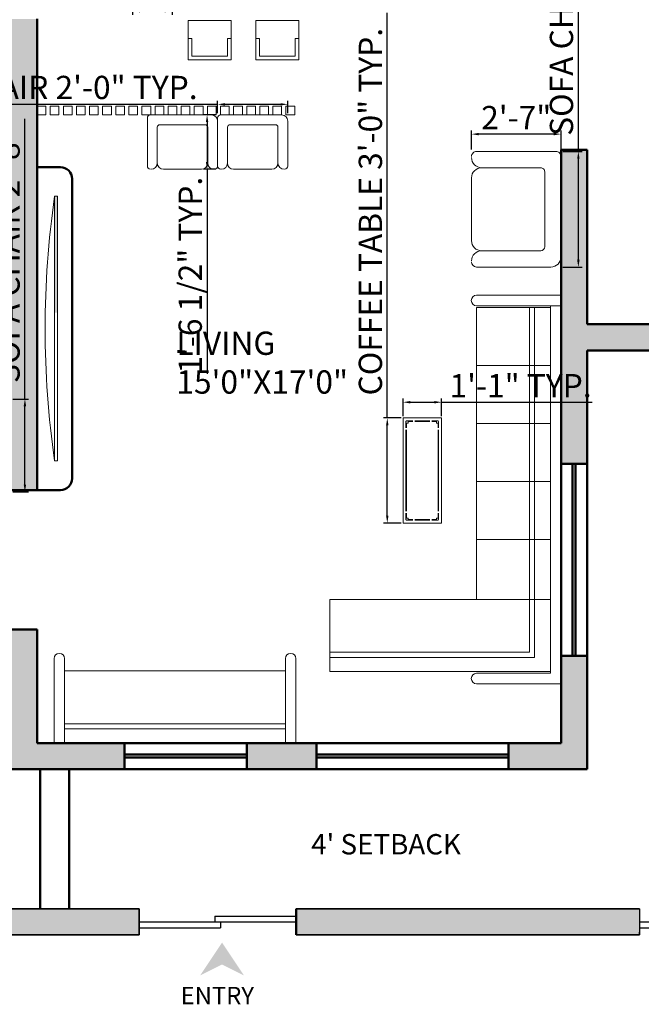
# Model space of a CAD drawing. Units: inches. Extents: x 2442 to 3851, y 589 to 2836.
# Tile 5 of 22: x 2698 to 2911, y 1378 to 1717. Entities that reach past the tile are written whole.
import ezdxf

# ---------------------------------------------------------------- set-up
doc = ezdxf.new("R2010")
doc.units = ezdxf.units.IN
for name, color, linetype, lineweight in [('A-ANNO-DIMS', 2, 'Continuous', 18), ('A-ANNO-SYMB', 1, 'Continuous', 18), ('A-ANNO-TEXT', 7, 'Continuous', 18), ('A-AREA-IDEN', 7, 'Continuous', 18), ('A-FURN', 8, 'Continuous', 18), ('A-GLAZ', 1, 'Continuous', 25), ('A-WALL', 7, 'Continuous', 50), ('A-WALL-PATT', 8, 'Continuous', 13), ('C-PROP', 7, 'Continuous', 35)]:
    doc.layers.add(name, color=color, linetype=linetype, lineweight=lineweight)
doc.styles.get("Standard").update_dxf_attribs({"font": 'arial.ttf'})
doc.dimstyles.new('ISO-25', dxfattribs={"dimtxt": 8, "dimasz": 2.5, "dimexe": 1.25, "dimexo": 0.625, "dimtad": 1, "dimlunit": 3, "dimtxsty": 'Standard', "dimcen": 2.5, "dimadec": 0, "dimazin": 0, "dimtfac": 1, "dimtmove": 0, "dimatfit": 3, "dimfxl": 1, "dimarcsym": 0})

# ---------------------------------------------------------------- blocks, each defined once
blk = doc.blocks.new('sofa-27')
at = {"color": 0, "linetype": 'ByBlock'}
for p, q in [((0.0945, 0.5198), (0.459, 0.5198)), ((-0.0591, 0.0591), (-0.0591, 0.4902)), ((0.0354, 0.1181), (0.0354, 0.4607)), ((0.518, 0.1181), (0.518, 0.4607)), ((0.6125, 0.0295), (0.6125, 0.4902)), ((0.4944, 0.0945), (0.0591, 0.0945)), ((0.583, 0), (0, 0))]:
    blk.add_line(p, q, dxfattribs=at)
for centre, radius, start, end in [((-0.0295, 0.4902), 0.0295, 90, 180), ((-0.0236, 0.4607), 0.0591, 360, 90), ((0.0945, 0.4607), 0.0591, 90, 180), ((0.459, 0.4607), 0.0591, 0, 90), ((0.5771, 0.4607), 0.0591, 90, 180), ((0.583, 0.4902), 0.0295, 0, 90), ((0.0591, 0.1181), 0.0236, 180, 270), ((0.4944, 0.1181), 0.0236, 270, 0), ((0, 0.0591), 0.0591, 180, 270), ((0.583, 0.0295), 0.0295, 270, 0)]:
    blk.add_arc(centre, radius, start, end, dxfattribs=at)
blk = doc.blocks.new('TABLE-30A')
at = {"color": 0, "linetype": 'ByBlock'}
for p, q in [((0, 0), (0, 0.55)), ((0, 0.55), (1.5, 0.55)), ((0.051, 0.508), (0.042, 0.499)), ((0.042, 0.499), (0.042, 0.478)), ((0.042, 0.478), (0.072, 0.478)), ((0.042, 0.478), (0.042, 0.41)), ((0.072, 0.508), (0.051, 0.508)), ((0.051, 0.478), (0.051, 0.41)), ((0.072, 0.478), (0.072, 0.508)), ((0.072, 0.508), (0.14, 0.508)), ((0.072, 0.499), (0.14, 0.499)), ((1.331, 0.508), (0.169, 0.508)), ((1.331, 0.499), (0.169, 0.499)), ((1.428, 0.508), (1.36, 0.508)), ((1.428, 0.499), (1.36, 0.499)), ((1.428, 0.508), (1.428, 0.478)), ((1.449, 0.508), (1.428, 0.508)), ((1.428, 0.478), (1.458, 0.478)), ((1.458, 0.499), (1.449, 0.508)), ((1.449, 0.478), (1.449, 0.41)), ((1.458, 0.478), (1.458, 0.499)), ((1.458, 0.478), (1.458, 0.41)), ((1.5, 0.55), (1.5, 0)), ((0.042, 0.169), (0.042, 0.381)), ((0.051, 0.169), (0.051, 0.381)), ((1.449, 0.381), (1.449, 0.169)), ((1.458, 0.381), (1.458, 0.169)), ((1.5, 0), (0, 0)), ((0.042, 0.072), (0.042, 0.14)), ((0.042, 0.072), (0.042, 0.051)), ((0.072, 0.072), (0.042, 0.072)), ((0.042, 0.051), (0.051, 0.042)), ((0.051, 0.072), (0.051, 0.14)), ((0.051, 0.042), (0.072, 0.042)), ((0.072, 0.042), (0.072, 0.072)), ((0.072, 0.051), (0.14, 0.051)), ((0.072, 0.042), (0.14, 0.042)), ((0.169, 0.051), (1.331, 0.051)), ((0.169, 0.042), (1.331, 0.042)), ((1.428, 0.051), (1.36, 0.051)), ((1.428, 0.042), (1.36, 0.042)), ((1.428, 0.072), (1.428, 0.042)), ((1.458, 0.072), (1.428, 0.072)), ((1.428, 0.042), (1.449, 0.042)), ((1.449, 0.072), (1.449, 0.14)), ((1.449, 0.042), (1.458, 0.051)), ((1.458, 0.072), (1.458, 0.14)), ((1.458, 0.051), (1.458, 0.072))]:
    blk.add_line(p, q, dxfattribs=at)
blk = doc.blocks.new('*U26')
at = {"linetype": 'ByBlock'}
blk.add_lwpolyline([(-1.5, -1.5), (1.5, -1.5), (1.5, 1.5), (-1.5, 1.5)], close=True, dxfattribs=at)
blk = doc.blocks.new('*U27')
at = {"layer": 'A-FURN', "color": 0, "linetype": 'ByBlock', "lineweight": -2, "transparency": 16777216}
for p in [(0, 0), (4.5, 0), (9, 0), (13.5, 0), (18, 0), (22.5, 0), (27, 0), (31.5, 0), (36, 0), (40.5, 0), (45, 0), (49.5, 0), (54, 0), (58.5, 0), (63, 0), (67.5, 0), (72, 0), (76.5, 0), (81, 0), (85.5, 0)]:
    blk.add_blockref('*U26', p, dxfattribs=at)
blk = doc.blocks.new('CHAIR-DINING')
for p, q in [((0, 14.84), (13.57, 14.84)), ((0, 0), (0, 14.84)), ((1.28, 13.56), (7.42, 13.56)), ((1.28, 1.32), (1.28, 13.56)), ((7.42, 13.56), (7.42, 14.84)), ((13.57, 0), (13.57, 14.84)), ((0, 0), (13.57, 0)), ((7.42, 1.32), (1.28, 1.32)), ((7.42, 0), (7.42, 1.32))]:
    blk.add_line(p, q)
blk = doc.blocks.new('SOFA-L')
for p, q in [((79.48, 133.62), (50.46, 133.62)), ((79.48, 0), (79.48, 133.62)), ((79.48, 129.99), (50.46, 129.99)), ((50.46, 129.38), (50.46, 29.02)), ((75.86, 129.38), (50.46, 129.38)), ((75.86, 129.38), (50.46, 129.38)), ((75.86, 3.63), (75.86, 129.99)), ((75.86, 29.02), (0, 29.02)), ((0, 4.23), (0, 29.02)), ((75.86, 4.23), (0, 4.23)), ((50.46, 3.63), (75.86, 3.63)), ((50.46, 0), (79.48, 0))]:
    blk.add_line(p, q)
for centre in [(50.46, 131.8), (50.46, 1.81)]:
    blk.add_arc(centre, 1.81, 90, 270)
blk = doc.blocks.new('SOFA-3SEAT')
for p, q in [((0, 29.02), (0, 0)), ((3.63, 0), (3.63, 29.02)), ((79.48, 29.02), (79.48, 0)), ((83.11, 29.02), (83.11, 0)), ((83.11, 0), (0, 0))]:
    blk.add_line(p, q)
for centre in [(1.81, 29.02), (81.3, 29.02)]:
    blk.add_arc(centre, 1.81, 0, 180)
blk = doc.blocks.new('*D149')
at = {"layer": 'A-ANNO-DIMS', "color": 0, "lineweight": -2, "transparency": 16777216}
for p, q in [((2736.38, 1721.15), (2736.38, 1718.3)), ((2749.95, 1721.15), (2749.95, 1718.3)), ((2738.88, 1719.55), (2747.45, 1719.55)), ((2749.95, 1719.55), (2820.35, 1719.55))]:
    blk.add_line(p, q, dxfattribs=at)
at = {"layer": 'A-ANNO-DIMS', "color": 0, "transparency": 16777216}
for points in [[(2738.88, 1719.96), (2738.88, 1719.13), (2736.38, 1719.55)], [(2747.45, 1719.96), (2747.45, 1719.13), (2749.95, 1719.55)]]:
    blk.add_solid(points, dxfattribs=at)
at = {"layer": 'Defpoints', "color": 0, "transparency": 16777216}
for p in [(2736.38, 1721.77), (2749.95, 1721.77), (2749.95, 1719.55)]:
    blk.add_point(p, dxfattribs=at)
at = {"layer": 'A-ANNO-DIMS', "color": 0, "transparency": 16777216, "insert": (2786.4, 1724.31), "char_height": 8, "attachment_point": 5}
blk.add_mtext('1\'-1 1/2" TYP.', dxfattribs=at)
blk = doc.blocks.new('*D150')
at = {"layer": 'A-ANNO-DIMS', "color": 0, "lineweight": -2, "transparency": 16777216}
for p, q in [((2699.39, 1586.16), (2699.39, 1682.55)), ((2695.22, 1586.16), (2700.64, 1586.16)), ((2699.39, 1556.72), (2699.39, 1583.66)), ((2695.22, 1554.22), (2700.64, 1554.22))]:
    blk.add_line(p, q, dxfattribs=at)
at = {"layer": 'A-ANNO-DIMS', "color": 0, "transparency": 16777216}
for points in [[(2698.97, 1583.66), (2699.81, 1583.66), (2699.39, 1586.16)], [(2698.97, 1556.72), (2699.81, 1556.72), (2699.39, 1554.22)]]:
    blk.add_solid(points, dxfattribs=at)
at = {"layer": 'Defpoints', "color": 0, "transparency": 16777216}
for p in [(2694.6, 1586.16), (2699.39, 1586.16), (2694.6, 1554.22)]:
    blk.add_point(p, dxfattribs=at)
at = {"layer": 'A-ANNO-DIMS', "color": 0, "transparency": 16777216, "insert": (2694.63, 1635.61), "char_height": 8, "attachment_point": 5, "rotation": 90}
blk.add_mtext('SOFA CHAIR 2\'-8"', dxfattribs=at)
blk = doc.blocks.new('*D152')
at = {"layer": 'A-ANNO-DIMS', "color": 0, "lineweight": -2, "transparency": 16777216}
for p, q in [((2889.56, 1671.28), (2889.56, 1786.31)), ((2884.22, 1671.28), (2890.81, 1671.28)), ((2889.56, 1634.03), (2889.56, 1668.78)), ((2884.22, 1631.53), (2890.81, 1631.53))]:
    blk.add_line(p, q, dxfattribs=at)
at = {"layer": 'A-ANNO-DIMS', "color": 0, "transparency": 16777216}
for points in [[(2889.14, 1668.78), (2889.98, 1668.78), (2889.56, 1671.28)], [(2889.14, 1634.03), (2889.98, 1634.03), (2889.56, 1631.53)]]:
    blk.add_solid(points, dxfattribs=at)
at = {"layer": 'Defpoints', "color": 0, "transparency": 16777216}
for p in [(2883.6, 1671.28), (2889.56, 1671.28), (2883.6, 1631.53)]:
    blk.add_point(p, dxfattribs=at)
at = {"layer": 'A-ANNO-DIMS', "color": 0, "transparency": 16777216, "insert": (2884.79, 1730.04), "char_height": 8, "attachment_point": 5, "rotation": 90}
blk.add_mtext('SOFA CHAIR 3\'-3 1/2"', dxfattribs=at)
blk = doc.blocks.new('*D153')
at = {"layer": 'A-ANNO-DIMS', "color": 0, "lineweight": -2, "transparency": 16777216}
for p, q in [((2852.84, 1671.9), (2852.84, 1678.49)), ((2881.1, 1677.24), (2855.34, 1677.24)), ((2883.6, 1671.9), (2883.6, 1678.49))]:
    blk.add_line(p, q, dxfattribs=at)
at = {"layer": 'A-ANNO-DIMS', "color": 0, "transparency": 16777216}
for points in [[(2855.34, 1677.66), (2855.34, 1676.82), (2852.84, 1677.24)], [(2881.1, 1677.66), (2881.1, 1676.82), (2883.6, 1677.24)]]:
    blk.add_solid(points, dxfattribs=at)
at = {"layer": 'Defpoints', "color": 0, "transparency": 16777216}
for p in [(2852.84, 1677.24), (2852.84, 1671.28), (2883.6, 1671.28)]:
    blk.add_point(p, dxfattribs=at)
at = {"layer": 'A-ANNO-DIMS', "color": 0, "transparency": 16777216, "insert": (2868.22, 1681.88), "char_height": 8, "attachment_point": 5}
blk.add_mtext('2\'-7"', dxfattribs=at)
blk = doc.blocks.new('*D154')
at = {"layer": 'A-ANNO-DIMS', "color": 0, "lineweight": -2, "transparency": 16777216}
for p, q in [((2765.6, 1687.48), (2641.71, 1687.48)), ((2765.6, 1684.49), (2765.6, 1688.73)), ((2787.22, 1687.48), (2768.1, 1687.48)), ((2789.72, 1684.49), (2789.72, 1688.73))]:
    blk.add_line(p, q, dxfattribs=at)
at = {"layer": 'A-ANNO-DIMS', "color": 0, "transparency": 16777216}
for points in [[(2768.1, 1687.9), (2768.1, 1687.07), (2765.6, 1687.48)], [(2787.22, 1687.9), (2787.22, 1687.07), (2789.72, 1687.48)]]:
    blk.add_solid(points, dxfattribs=at)
at = {"layer": 'Defpoints', "color": 0, "transparency": 16777216}
for p in [(2765.6, 1687.48), (2765.6, 1683.86), (2789.72, 1683.86)]:
    blk.add_point(p, dxfattribs=at)
at = {"layer": 'A-ANNO-DIMS', "color": 0, "transparency": 16777216, "insert": (2702.4, 1692.25), "char_height": 8, "attachment_point": 5}
blk.add_mtext('SOFA CHAIR 2\'-0" TYP.', dxfattribs=at)
blk = doc.blocks.new('*D155')
at = {"layer": 'A-ANNO-DIMS', "color": 0, "lineweight": -2, "transparency": 16777216}
for p, q in [((2764.97, 1683.86), (2760.73, 1683.86)), ((2761.98, 1681.36), (2761.98, 1667.69)), ((2764.97, 1665.19), (2760.73, 1665.19)), ((2761.98, 1665.19), (2761.98, 1594.79))]:
    blk.add_line(p, q, dxfattribs=at)
at = {"layer": 'A-ANNO-DIMS', "color": 0, "transparency": 16777216}
for points in [[(2761.56, 1681.36), (2762.4, 1681.36), (2761.98, 1683.86)], [(2761.56, 1667.69), (2762.4, 1667.69), (2761.98, 1665.19)]]:
    blk.add_solid(points, dxfattribs=at)
at = {"layer": 'Defpoints', "color": 0, "transparency": 16777216}
for p in [(2765.6, 1683.86), (2761.98, 1665.19), (2765.6, 1665.19)]:
    blk.add_point(p, dxfattribs=at)
at = {"layer": 'A-ANNO-DIMS', "color": 0, "transparency": 16777216, "insert": (2757.22, 1628.74), "char_height": 8, "attachment_point": 5, "rotation": 90}
blk.add_mtext('1\'-6 1/2" TYP.', dxfattribs=at)
blk = doc.blocks.new('*D166')
at = {"layer": 'A-ANNO-DIMS', "color": 0, "lineweight": -2, "transparency": 16777216}
for p, q in [((2823.9, 1579.64), (2823.9, 1719)), ((2828.69, 1579.64), (2822.65, 1579.64)), ((2823.9, 1546), (2823.9, 1577.14)), ((2828.69, 1543.5), (2822.65, 1543.5))]:
    blk.add_line(p, q, dxfattribs=at)
at = {"layer": 'A-ANNO-DIMS', "color": 0, "transparency": 16777216}
for points in [[(2823.48, 1577.14), (2824.31, 1577.14), (2823.9, 1579.64)], [(2823.48, 1546), (2824.31, 1546), (2823.9, 1543.5)]]:
    blk.add_solid(points, dxfattribs=at)
at = {"layer": 'Defpoints', "color": 0, "transparency": 16777216}
for p in [(2823.9, 1579.64), (2829.32, 1579.64), (2829.32, 1543.5)]:
    blk.add_point(p, dxfattribs=at)
at = {"layer": 'A-ANNO-DIMS', "color": 0, "transparency": 16777216, "insert": (2819.13, 1650.57), "char_height": 8, "attachment_point": 5, "rotation": 90}
blk.add_mtext('COFFEE TABLE 3\'-0" TYP.', dxfattribs=at)
blk = doc.blocks.new('*D167')
at = {"layer": 'A-ANNO-DIMS', "color": 0, "lineweight": -2, "transparency": 16777216}
for p, q in [((2829.32, 1580.26), (2829.32, 1586.31)), ((2831.82, 1585.06), (2840.07, 1585.06)), ((2842.57, 1580.26), (2842.57, 1586.31)), ((2842.57, 1585.06), (2894.33, 1585.06))]:
    blk.add_line(p, q, dxfattribs=at)
at = {"layer": 'A-ANNO-DIMS', "color": 0, "transparency": 16777216}
for points in [[(2831.82, 1585.47), (2831.82, 1584.64), (2829.32, 1585.06)], [(2840.07, 1585.47), (2840.07, 1584.64), (2842.57, 1585.06)]]:
    blk.add_solid(points, dxfattribs=at)
at = {"layer": 'Defpoints', "color": 0, "transparency": 16777216}
for p in [(2842.57, 1585.06), (2829.32, 1579.64), (2842.57, 1579.64)]:
    blk.add_point(p, dxfattribs=at)
at = {"layer": 'A-ANNO-DIMS', "color": 0, "transparency": 16777216, "insert": (2869.7, 1589.7), "char_height": 8, "attachment_point": 5}
blk.add_mtext('1\'-1" TYP.', dxfattribs=at)

msp = doc.modelspace()

# ---------------------------------------------------------------- hatches: boundary and pattern name
at = {"layer": 'A-ANNO-SYMB'}
h = msp.add_hatch(color=256, dxfattribs=at)
h.dxf.hatch_style = 1
h.paths.add_polyline_path([(2767.136, 1391.705), (2774.686, 1387.93), (2767.136, 1399.256), (2759.585, 1387.93)])
at = {"layer": 'A-FURN'}
h = msp.add_hatch(color=256, dxfattribs=at)
h.dxf.hatch_style = 1
h.paths.add_polyline_path([(2710.599, 1655.864), (2709.599, 1655.864), (2709.599, 1615.864), (2710.599, 1615.864)])
at = {"layer": 'A-WALL-PATT'}
h = msp.add_hatch(color=256, dxfattribs=at)
h.dxf.hatch_style = 1
h.paths.add_polyline_path([(2502.599, 1992.864), (2719.571, 1992.864), (2719.687, 1994.649), (2720.167, 1997.319), (2721.479, 1992.864), (2726.325, 1992.864), (2727.448, 1994.93), (2729.005, 1997.153), (2728.372, 1992.864), (2728.871, 1992.864), (2730.114, 1994.505), (2731.833, 1996.09), (2730.966, 1993.206), (2730.864, 1992.864), (2771.772, 1992.864), (2771.887, 1994.649), (2772.368, 1997.319), (2773.68, 1992.864), (2778.526, 1992.864), (2779.649, 1994.93), (2781.206, 1997.153), (2780.572, 1992.864), (2781.072, 1992.864), (2782.315, 1994.505), (2784.034, 1996.09), (2783.167, 1993.206), (2783.065, 1992.864), (2821.282, 1992.864), (2821.398, 1994.649), (2821.878, 1997.319), (2823.19, 1992.864), (2828.036, 1992.864), (2829.159, 1994.93), (2830.716, 1997.153), (2830.083, 1992.864), (2830.582, 1992.864), (2831.825, 1994.505), (2833.544, 1996.09), (2832.677, 1993.206), (2832.575, 1992.864), (2869.287, 1992.864), (2869.403, 1994.649), (2869.884, 1997.319), (2871.195, 1992.864), (2876.042, 1992.864), (2877.165, 1994.93), (2878.721, 1997.153), (2878.088, 1992.864), (2878.587, 1992.864), (2879.83, 1994.505), (2881.55, 1996.09), (2880.682, 1993.206), (2880.58, 1992.864), (2919.335, 1992.864), (2919.451, 1994.649), (2919.932, 1997.319), (2921.243, 1992.864), (2926.09, 1992.864), (2927.213, 1994.93), (2928.77, 1997.153), (2928.136, 1992.864), (2928.635, 1992.864), (2929.878, 1994.505), (2931.598, 1996.09), (2930.73, 1993.206), (2930.628, 1992.864), (2966.155, 1992.864), (2966.27, 1994.649), (2966.751, 1997.319), (2968.063, 1992.864), (2972.909, 1992.864), (2974.032, 1994.93), (2975.589, 1997.153), (2974.955, 1992.864), (2975.455, 1992.864), (2976.698, 1994.505), (2978.417, 1996.09), (2977.55, 1993.206), (2977.448, 1992.864), (3010.53, 1992.864), (3010.646, 1994.649), (3011.127, 1997.319), (3012.438, 1992.864), (3017.285, 1992.864), (3018.408, 1994.93), (3019.964, 1997.153), (3019.331, 1992.864), (3019.83, 1992.864), (3021.073, 1994.505), (3022.793, 1996.09), (3021.925, 1993.206), (3021.823, 1992.864), (3057.996, 1992.864), (3058.45, 1995.382), (3059.191, 1992.864), (3065.64, 1992.864), (3067.287, 1995.216), (3066.94, 1992.864), (3068.717, 1992.864), (3070.116, 1994.153), (3069.728, 1992.864), (3084.599, 1992.864), (3084.599, 1983.791), (3085.291, 1983.828), (3084.599, 1983.434), (3084.599, 1932.114), (3085.291, 1932.151), (3084.599, 1931.757), (3084.599, 1886.278), (3085.291, 1886.315), (3084.599, 1885.921), (3084.599, 1410.864), (3066.599, 1410.864), (3066.599, 1401.864), (3093.599, 1401.864), (3093.599, 2001.864), (2493.599, 2001.864), (2493.599, 1401.864), (2538.599, 1401.864), (2538.599, 1410.864), (2502.599, 1410.864)])
h.paths.add_polyline_path([(2738.599, 1410.864), (2547.599, 1410.864), (2547.599, 1401.864), (2738.599, 1401.864)], flags=17)
h.paths.add_polyline_path([(2910.599, 1410.864), (2792.599, 1410.864), (2792.599, 1401.864), (2910.599, 1401.864), (2910.599, 1402.864)], flags=17)
h = msp.add_hatch(color=256, dxfattribs=at)
h.dxf.hatch_style = 1
h.paths.add_polyline_path([(2799.599, 1467.864), (2775.599, 1467.864), (2775.599, 1458.864), (2799.599, 1458.864)])
h.paths.add_polyline_path([(2703.599, 1506.864), (2670.599, 1506.864), (2670.599, 1497.864), (2694.599, 1497.864), (2694.599, 1458.864), (2733.599, 1458.864), (2733.599, 1467.864), (2709.417, 1467.864), (2703.599, 1467.864)])
h.paths.add_polyline_path([(2604.599, 1506.864), (2593.599, 1506.864), (2593.599, 1497.864), (2604.599, 1497.864)])
h.paths.add_polyline_path([(2547.599, 1497.864), (2553.599, 1497.864), (2553.599, 1506.864), (2547.599, 1506.864), (2547.599, 1530.864), (2538.599, 1530.864), (2538.599, 1401.864), (2547.599, 1401.864)])
h.paths.add_polyline_path([(2547.599, 1683.864), (2538.599, 1683.864), (2538.599, 1578.864), (2547.599, 1578.864), (2547.599, 1602.864), (2694.599, 1602.864), (2694.599, 1554.864), (2703.599, 1554.864), (2703.599, 1716.864), (2694.599, 1716.864), (2694.599, 1611.864), (2547.599, 1611.864)])
h.paths.add_polyline_path([(2892.599, 1497.864), (2883.599, 1497.864), (2883.599, 1488.228), (2883.599, 1467.864), (2865.599, 1467.864), (2865.599, 1458.864), (2892.599, 1458.864)])
h.paths.add_polyline_path([(3048.599, 1722.864), (3039.599, 1722.864), (3039.599, 1716.864), (2937.599, 1716.864), (2937.599, 1710.864), (3039.599, 1710.864), (3039.599, 1685.364), (3048.599, 1685.364)])
h.paths.add_polyline_path([(3048.599, 1779.864), (3039.599, 1779.864), (3039.599, 1773.864), (2961.599, 1773.864), (2961.599, 1791.864), (2955.599, 1791.864), (2955.599, 1773.864), (2895.599, 1773.864), (2895.599, 1821.864), (2916.599, 1821.864), (2916.599, 1827.864), (2889.599, 1827.864), (2889.599, 1773.864), (2886.599, 1773.864), (2886.599, 1764.864), (2937.599, 1764.864), (2937.599, 1746.864), (2943.599, 1746.864), (2943.599, 1764.864), (2956.06, 1764.864), (3039.599, 1764.864), (3039.599, 1758.864), (3048.599, 1758.864)])
h.paths.add_polyline_path([(3048.599, 1827.864), (2976.475, 1827.864, -0.1284593), (2975.705, 1827.665), (2964.694, 1827.687, -0.1198794), (2963.972, 1827.864), (2946.599, 1827.864), (2946.599, 1821.864), (3039.599, 1821.864), (3039.599, 1815.864), (3048.599, 1815.864)])
h.paths.add_polyline_path([(3048.599, 1956.864), (3023.366, 1956.864), (3023.277, 1956.402), (3023.088, 1956.864), (3019.494, 1956.864), (3019.543, 1955.479), (3019.146, 1956.864), (3015.599, 1956.864), (3015.599, 1947.864), (3039.599, 1947.864), (3039.599, 1875.864), (3048.599, 1875.864), (3048.599, 1880.743), (3047.576, 1881.614), (3046.081, 1883.417), (3044.931, 1885.453), (3047.541, 1883.949), (3048.599, 1883.343), (3048.599, 1910.588), (3047.049, 1909.235), (3047.896, 1910.862), (3048.599, 1911.909), (3048.599, 1918.826), (3042.477, 1917.032), (3043.928, 1918.154), (3045.59, 1919.165), (3047.525, 1920.009), (3048.599, 1920.305), (3048.599, 1926.579), (3047.576, 1927.45), (3046.081, 1929.252), (3044.931, 1931.289), (3047.541, 1929.785), (3048.599, 1929.179)])
h.paths.add_polyline_path([(2967.599, 1956.864), (2932.171, 1956.864), (2932.082, 1956.402), (2931.893, 1956.864), (2928.299, 1956.864), (2928.348, 1955.479), (2927.951, 1956.864), (2898.599, 1956.864), (2898.599, 1947.864), (2967.599, 1947.864)])
h.paths.add_polyline_path([(2850.599, 1956.864), (2834.118, 1956.864), (2834.029, 1956.402), (2833.84, 1956.864), (2830.245, 1956.864), (2830.294, 1955.479), (2829.897, 1956.864), (2796.599, 1956.864), (2796.599, 1947.864), (2799.599, 1947.864), (2838.599, 1947.864), (2838.599, 1827.864), (2835.599, 1827.864), (2835.599, 1824.864), (2835.599, 1818.864), (2838.599, 1818.864), (2838.599, 1764.864), (2850.599, 1764.864), (2850.599, 1770.864), (2850.599, 1773.864), (2847.599, 1773.864), (2847.599, 1947.864), (2850.599, 1947.864)])
h.paths.add_polyline_path([(2700.599, 1947.864), (2730.599, 1947.864), (2730.599, 1956.864), (2700.599, 1956.864), (2700.599, 1992.864), (2691.599, 1992.864), (2691.599, 1932.864), (2670.599, 1932.864), (2670.599, 1923.864), (2691.599, 1923.864), (2691.599, 1818.864), (2799.599, 1818.864), (2799.599, 1827.864), (2700.599, 1827.864)])
h.paths.add_polyline_path([(2640.599, 1932.864), (2538.599, 1932.864), (2538.599, 1868.364), (2547.599, 1868.364), (2547.599, 1923.864), (2640.599, 1923.864), (2640.599, 1929.864)])
h.paths.add_polyline_path([(2547.599, 1820.364), (2538.599, 1820.364), (2538.599, 1731.864), (2547.599, 1731.864), (2547.599, 1755.864), (2694.599, 1755.864), (2694.599, 1752.864), (2697.599, 1752.864), (2703.599, 1752.864), (2703.599, 1764.864), (2547.599, 1764.864)])
h.paths.add_polyline_path([(2725.858, 1838.187), (2790.115, 1838.187), (2790.115, 1868.602), (2725.858, 1868.602)], flags=25)
h.paths.add_polyline_path([(2892.599, 1671.864), (2883.599, 1671.864), (2883.599, 1563.864), (2892.599, 1563.864), (2892.599, 1602.864), (3048.599, 1602.864), (3048.599, 1637.364), (3039.599, 1637.364), (3039.599, 1611.864), (2892.599, 1611.864)])

# ---------------------------------------------------------------- linework, layer by layer
at = {"layer": 'A-FURN'}
for p, q in [((2709.599, 1655.864), (2710.599, 1655.864)), ((2709.599, 1564.864), (2709.599, 1655.864)), ((2710.599, 1564.864), (2710.599, 1655.864)), ((2872.716, 1499.111), (2872.716, 1617.612)), ((2874.53, 1497.297), (2874.53, 1617.612)), ((2879.971, 1597.66), (2854.577, 1597.66)), ((2879.971, 1577.709), (2854.577, 1577.709)), ((2709.599, 1564.864), (2710.599, 1564.864)), ((2879.971, 1557.758), (2854.577, 1557.758)), ((2879.971, 1537.806), (2854.577, 1537.806)), ((2804.116, 1499.111), (2872.716, 1499.111)), ((2804.116, 1497.297), (2874.53, 1497.297)), ((2788.9, 1492.651), (2713.045, 1492.651)), ((2713.045, 1474.513), (2788.9, 1474.513)), ((2713.045, 1472.699), (2788.9, 1472.699))]:
    msp.add_line(p, q, dxfattribs=at)
msp.add_arc((3023.084, 1610.364), 316.77, 171.74163, 188.25837, dxfattribs=at)
at = {"layer": 'A-GLAZ'}
for p, q in [((2910.599, 1410.864), (2910.599, 1401.864)), ((2738.599, 1406.364), (2792.599, 1406.364)), ((2764.599, 1408.364), (2792.599, 1408.364)), ((2764.599, 1408.364), (2764.599, 1406.364)), ((2766.599, 1406.364), (2766.599, 1404.364)), ((2910.599, 1406.364), (3066.599, 1406.364)), ((2738.599, 1404.364), (2766.599, 1404.364)), ((2910.599, 1404.364), (2989.599, 1404.364)), ((2910.599, 1401.864), (2910.599, 1402.864))]:
    msp.add_line(p, q, dxfattribs=at)
at = {"layer": 'A-WALL'}
for p, q in [((2703.599, 1554.864), (2703.599, 1716.864)), ((2883.599, 1467.864), (2883.599, 1671.864)), ((2883.599, 1671.864), (2892.599, 1671.864)), ((2892.599, 1611.864), (2892.599, 1671.864)), ((2703.599, 1665.864), (2711.599, 1665.864)), ((2703.599, 1605.864), (2703.599, 1665.864)), ((2715.599, 1661.864), (2715.599, 1558.864)), ((2892.599, 1611.864), (3039.599, 1611.864)), ((2892.599, 1458.864), (2892.599, 1602.864)), ((2892.599, 1602.864), (3048.599, 1602.864)), ((2883.599, 1563.864), (2892.599, 1563.864)), ((2887.599, 1497.864), (2887.599, 1563.864)), ((2888.599, 1497.864), (2888.599, 1563.864)), ((2694.599, 1554.864), (2703.599, 1554.864)), ((2703.599, 1554.864), (2711.599, 1554.864)), ((2593.599, 1506.864), (2703.599, 1506.864)), ((2703.599, 1467.864), (2703.599, 1506.864)), ((2883.599, 1497.864), (2892.599, 1497.864)), ((2703.599, 1467.864), (2883.599, 1467.864)), ((2733.599, 1458.864), (2733.599, 1467.864)), ((2775.599, 1458.864), (2775.599, 1467.864)), ((2799.599, 1458.864), (2799.599, 1467.864)), ((2865.599, 1458.864), (2865.599, 1467.864)), ((2733.599, 1463.864), (2775.599, 1463.864)), ((2733.599, 1462.864), (2775.599, 1462.864)), ((2799.599, 1463.864), (2865.599, 1463.864)), ((2799.599, 1462.864), (2865.599, 1462.864)), ((2694.599, 1458.864), (2892.599, 1458.864)), ((2704.599, 1410.864), (2704.599, 1458.864)), ((2714.599, 1410.864), (2714.599, 1458.864)), ((2792.599, 1401.864), (2792.599, 1410.864))]:
    msp.add_line(p, q, dxfattribs=at)
for centre, start, end in [((2711.599, 1661.864), 0, 90), ((2711.599, 1558.864), 270, 0)]:
    msp.add_arc(centre, 4, start, end, dxfattribs=at)
at = {"layer": 'C-PROP'}
msp.add_line((2738.599, 1401.864), (2738.599, 1410.864), dxfattribs=at)
for points in [[(3066.599, 1401.864), (3093.599, 1401.864), (3093.599, 2001.864), (2493.599, 2001.864), (2493.599, 1401.864), (2738.599, 1401.864)], [(2547.599, 1410.864), (2738.599, 1410.864)], [(2792.599, 1410.864), (2910.599, 1410.864)], [(2792.599, 1401.864), (2910.599, 1401.864)]]:
    msp.add_lwpolyline(points, dxfattribs=at)

# ---------------------------------------------------------------- block references
at = {"layer": 'A-FURN'}
for p, rotation in [((2770.275, 1702.744), 90.03023468100973), ((2793.523, 1702.741), 90.01148952388232)]:
    msp.add_blockref('CHAIR-DINING', p, dxfattribs=dict(at, rotation=rotation))
for name, p in [('*U27', (2705.099, 1685.364)), ('SOFA-L', (2804.116, 1488.228)), ('SOFA-3SEAT', (2709.417, 1467.864))]:
    msp.add_blockref(name, p, dxfattribs=at)
for name, p, xscale, yscale, zscale, rotation in [('sofa-27', (2763.476, 1683.864), 35.91933807128723, 35.91933807128723, 35.91933807128723, 179.9999999999668), ('sofa-27', (2787.599, 1683.864), 35.91933807128723, 35.91933807128723, 35.91933807128723, 179.9999999999668), ('sofa-27', (2883.599, 1635.029), 59.17827105340016, 59.17827105340016, 59.17827105340016, 89.9999999999668), ('TABLE-30A', (2829.318, 1543.504), -24.08863485716172, 24.08863485716172, 24.08863485716172, 270)]:
    msp.add_blockref(name, p, dxfattribs=dict(at, xscale=xscale, yscale=yscale, zscale=zscale, rotation=rotation))

# ---------------------------------------------------------------- texts
at = {"layer": 'A-ANNO-TEXT', "attachment_point": 1}
for s, width, insert, char_height in [("{\\fTimes New Roman|b0|i0|c0|p18;4' SETBACK}", 79.56037, (2797.738, 1436.558), 7), ('{\\fTimes New Roman|b0|i0|c0|p18;ENTRY}', 196.26071, (2752.918, 1384.023), 6)]:
    msp.add_mtext_dynamic_manual_height_columns(s, width=width, gutter_width=12.5, heights=[0], dxfattribs=dict(at, insert=insert, char_height=char_height))
at = {"layer": 'A-AREA-IDEN', "insert": (2751.422, 1609.338), "char_height": 8, "attachment_point": 1}
msp.add_mtext_dynamic_manual_height_columns('{\\fTimes New Roman|b0|i0|c0|p18;LIVING\\P15\'0"X17\'0"}', width=110.76054, gutter_width=12.5, heights=[0], dxfattribs=at)

# ---------------------------------------------------------------- dimensions: what is measured, and where the dimension line sits
at = {"layer": 'A-ANNO-DIMS'}
for base, p1, p2, angle, text, picture, middle in [((2889.56, 1671.277), (2883.599, 1631.534), (2883.599, 1671.277), 90, 'SOFA CHAIR <>', '*D152', (2884.793, 1730.042)), ((2765.598, 1687.482), (2789.72, 1683.864), (2765.598, 1683.864), 180, 'SOFA CHAIR <> TYP.', '*D154', (2702.404, 1692.247)), ((2823.898, 1579.637), (2829.318, 1543.504), (2829.318, 1579.637), 90, 'COFFEE TABLE <> TYP.', '*D166', (2819.131, 1650.568)), ((2761.979, 1665.195), (2765.598, 1683.864), (2765.598, 1665.195), 270, '<> TYP.', '*D155', (2757.218, 1628.744)), ((2699.39, 1586.162), (2694.599, 1554.22), (2694.599, 1586.162), 90, 'SOFA CHAIR <>', '*D150', (2694.626, 1635.606))]:
    dim = msp.add_linear_dim(base=base, p1=p1, p2=p2, angle=angle, text=text, dimstyle='ISO-25', override={"dimdec": 1, "dimrnd": 0, "dimzin": 1, "dimlunit": 4, "dimfrac": 2}, dxfattribs=at)
    dim.commit()
    dim.dimension.update_dxf_attribs({"geometry": picture, "text_midpoint": middle})
for base, p1, p2, picture, middle in [((2749.951, 1719.546), (2736.383, 1721.771), (2749.951, 1721.771), '*D149', (2786.402, 1724.307)), ((2842.567, 1585.057), (2829.318, 1579.637), (2842.567, 1579.637), '*D167', (2869.697, 1589.701))]:
    dim = msp.add_linear_dim(base=base, p1=p1, p2=p2, text='<> TYP.', dimstyle='ISO-25', override={"dimdec": 1, "dimrnd": 0, "dimzin": 1, "dimlunit": 4, "dimfrac": 2}, dxfattribs=at)
    dim.commit()
    dim.dimension.update_dxf_attribs({"geometry": picture, "text_midpoint": middle})
dim = msp.add_linear_dim(base=(2852.841, 1677.239), p1=(2883.599, 1671.277), p2=(2852.841, 1671.277), angle=180, dimstyle='ISO-25', override={"dimdec": 1, "dimrnd": 0, "dimzin": 1, "dimlunit": 4, "dimfrac": 2}, dxfattribs=at)
dim.commit()
dim.dimension.update_dxf_attribs({"geometry": '*D153', "text_midpoint": (2868.22, 1681.88)})

doc.saveas('drawing.dxf')
